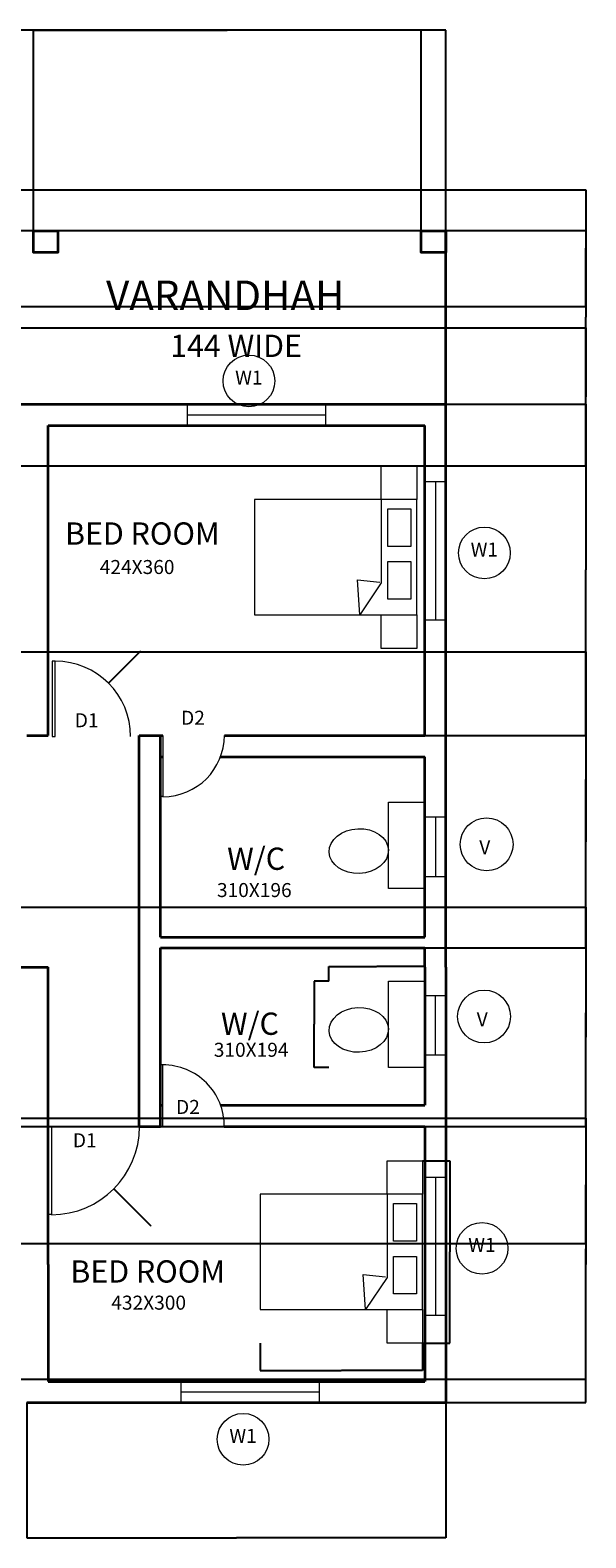
# Model space of a CAD drawing. Units: millimetres. Extents: x -2968 to 14333, y -2966 to 13411.
# Tile 3 of 3: x 8301 to 14333, y -2966 to 13411. Entities that reach past the tile are written whole.
import ezdxf

# ---------------------------------------------------------------- set-up
doc = ezdxf.new("R2010")
doc.units = ezdxf.units.MM
doc.header["$MEASUREMENT"] = 0
for name, color, linetype, lineweight in [('A-ANNO-DIMS', 2, 'Continuous', 18), ('A-ANNO-SYMB', 3, 'Continuous', 13), ('A-AREA-IDEN', 7, 'Continuous', 18), ('A-COLS', 7, 'Continuous', 35), ('A-DOOR', 3, 'Continuous', 18), ('A-FLOR-EDGE', 7, 'Continuous', 25), ('A-FLOR-FIXT', 9, 'Continuous', 18), ('A-FURN', 8, 'Continuous', 18), ('A-GLAZ', 4, 'Continuous', 18), ('A-WALL', 7, 'Continuous', 35)]:
    doc.layers.add(name, color=color, linetype=linetype, lineweight=lineweight)
doc.styles.get("Standard").update_dxf_attribs({"font": 'arial.ttf'})
doc.dimstyles.get("Standard").update_dxf_attribs({"dimtxt": 0.18, "dimasz": 0.18, "dimexe": 0.18, "dimexo": 0.0625, "dimgap": 0.09, "dimtad": 0, "dimtih": 1, "dimtoh": 1, "dimdec": 4, "dimzin": 0, "dimdsep": 46, "dimtxsty": 'Standard', "dimcen": 0.09, "dimadec": 0, "dimazin": 0, "dimtfac": 1, "dimtdec": 4, "dimtofl": 0, "dimtmove": 0, "dimatfit": 3, "dimfxl": 1, "dimtolj": 1, "dimtzin": 0, "dimarcsym": 0})

# ---------------------------------------------------------------- blocks, each defined once
blk = doc.blocks.new('DOOR-SWING-666')
blk.add_lwpolyline([(666.2992070210612, -7.87249337009e-05), (666.2992070210612, 666.0645318323222), (692.9797223629398, 666.0645318323222), (692.9797223629398, -7.87249337009e-05)], close=True)
blk.add_arc((666.2992070210612, -7.87249337009e-05), 666.2995763929106, 90, 180)
blk = doc.blocks.new('WIN-1500')
for p, q in [((-0.0001454069465439, 230.0001364428754), (-0.0001454069465439, 0.0001364428753732)), ((1499.999854593053, 230.0001364428754), (1499.999854593053, 0.0001364428753732)), ((-0.0001454069465439, 115.0001364428753), (1499.999854593053, 115.0001364428753))]:
    blk.add_line(p, q)
blk = doc.blocks.new('WIN-645')
for p, q in [((-0.0001783325678844, 645.3165217330161), (229.9998216674321, 645.3165217330161)), ((114.9998216674321, 645.3165217330161), (114.9998216674321, 9.39247611313e-05)), ((-0.0001783325678844, 9.39247611313e-05), (229.9998216674321, 9.39247611313e-05))]:
    blk.add_line(p, q)
blk = doc.blocks.new('BED-DOUBLE')
for points in [[(1376.583165448723, 1980.905007667385), (1761.472025135164, 1980.905007667385), (1761.472025135164, 1615.931306586089), (1376.583165448723, 1615.931306586089)], [(1761.359434948168, 1616.313451531646), (-6.24364656687e-05, 1616.313451531646), (-6.24364656687e-05, 364.9736316857862), (1761.359434948168, 364.9736316857862)], [(1446.690711967745, 1514.551870762266), (1696.927267861651, 1514.551870762266), (1696.927267861651, 1106.656997559254), (1446.690711967745, 1106.656997559254)], [(1446.690711967745, 942.1830025459176), (1696.927267861651, 942.1830025459176), (1696.927267861651, 534.2881293429062), (1446.690711967745, 534.2881293429062)], [(1376.470575261726, 364.9736316857862), (1761.359434948168, 364.9736316857862), (1761.359434948168, -6.93955107636e-05), (1376.470575261726, -6.93955107636e-05)]]:
    blk.add_lwpolyline(points, close=True)
blk.add_lwpolyline([(1376.583165448723, 1615.931306586089), (1376.583165448723, 711.9201034350671), (1143.773068517777, 363.235888262815), (1117.43252473963, 744.8148033080624), (1361.083249688014, 718.4988451502986)])
blk = doc.blocks.new('WC-PLAN')
blk.add_lwpolyline([(642.4076574105184, 937.925733504826), (1037.697987841055, 937.925733504826), (1037.697987841055, -0.0002773242667899), (642.4076574105184, -0.0002773242667899)], close=True)
blk.add_ellipse((321.2351413435845, 407.2568367539133), major_axis=(321.1725160669339, 12.34114489481309), ratio=0.7569293268408676)
blk = doc.blocks.new('VERANDAH-POST')
blk.add_lwpolyline([(-5.84108229305e-05, 235.3216454025205), (266.2404368537072, 235.3216454025205), (266.2404368537072, -0.0003482651118247), (-5.84108229305e-05, -0.0003482651118247)], close=True)
blk = doc.blocks.new('TAG-V')
blk.add_circle((287.0007825742364, 287.0011250592761), 287.0011736728098)
blk.add_text('V', height=152.3112078732942).set_placement((207.0741385544538, 179.2396726004772))
blk = doc.blocks.new('TAG-W1')
blk.add_circle((280.793431040287, 280.7932079668344), 280.7929963504647)
blk.add_text('W1', height=152.3112078732942).set_placement((130.9915239926576, 241.6268535788358))
blk = doc.blocks.new('*D20')
at = {"layer": 'A-ANNO-DIMS', "color": 0, "lineweight": -2, "transparency": 16777216}
for p, q in [((12560.39380992973, 1130.204523981605), (12857.64707148917, 1130.204523981605)), ((12857.46707148917, 1130.024523981605), (12857.46707148917, 139.9351164187788)), ((12857.46707148917, -850.5205530812917), (12857.46707148917, 139.5688544815346)), ((12560.39380992973, -850.7005530812916), (12857.64707148917, -850.7005530812916))]:
    blk.add_line(p, q, dxfattribs=at)
at = {"layer": 'A-ANNO-DIMS', "color": 0, "transparency": 16777216}
for points in [[(12857.43707148917, 1130.024523981605), (12857.49707148917, 1130.024523981605), (12857.46707148917, 1130.204523981605)], [(12857.43707148917, -850.5205530812917), (12857.49707148917, -850.5205530812917), (12857.46707148917, -850.7005530812916)]]:
    blk.add_solid(points, dxfattribs=at)
at = {"layer": 'Defpoints', "color": 0, "transparency": 16777216}
for p in [(12560.33130992973, 1130.204523981605), (12857.46707148917, 1130.204523981605), (12560.33130992973, -850.7005530812916)]:
    blk.add_point(p, dxfattribs=at)
at = {"layer": 'A-ANNO-DIMS', "color": 0, "transparency": 16777216, "insert": (12857.46707148917, 139.751985450153), "char_height": 0.18, "attachment_point": 5}
blk.add_mtext('\\A1;DOUBLE BED 1981 TYP.', dxfattribs=at)
blk = doc.blocks.new('*D21')
at = {"layer": 'A-ANNO-DIMS', "color": 0, "lineweight": -2, "transparency": 16777216}
for p, q in [((10798.85922235809, -850.7630530812912), (10798.85922235809, -1148.016314640725)), ((12560.33130992972, -850.7630530812912), (12560.33130992972, -1148.016314640725)), ((10799.03922235809, -1147.836314640725), (11678.93579820393, -1147.836314640725)), ((12560.15130992972, -1147.836314640725), (11680.25473408388, -1147.836314640725))]:
    blk.add_line(p, q, dxfattribs=at)
at = {"layer": 'A-ANNO-DIMS', "color": 0, "transparency": 16777216}
for points in [[(10799.03922235809, -1147.806314640725), (10799.03922235809, -1147.866314640725), (10798.85922235809, -1147.836314640725)], [(12560.15130992972, -1147.806314640725), (12560.15130992972, -1147.866314640725), (12560.33130992972, -1147.836314640725)]]:
    blk.add_solid(points, dxfattribs=at)
at = {"layer": 'Defpoints', "color": 0, "transparency": 16777216}
for p in [(10798.85922235809, -850.7005530812913), (12560.33130992972, -850.7005530812913), (12560.33130992972, -1147.836314640725)]:
    blk.add_point(p, dxfattribs=at)
at = {"layer": 'A-ANNO-DIMS', "color": 0, "transparency": 16777216, "insert": (11679.59526614391, -1147.836314640725), "char_height": 0.18, "attachment_point": 5}
blk.add_mtext('\\A1;1761 TYP.', dxfattribs=at)
blk = doc.blocks.new('*D28')
at = {"layer": 'A-ANNO-DIMS', "color": 0, "lineweight": -2, "transparency": 16777216}
for p, q in [((11541.92952659912, 3081.768817646303), (11541.92952659912, 3238.305486832592)), ((11542.10952659912, 3238.125486832593), (12062.41073402773, 3238.125486832593)), ((12584.54398784105, 3238.125486832593), (12064.24278041245, 3238.125486832593)), ((12584.72398784105, 3081.768817646303), (12584.72398784105, 3238.305486832592))]:
    blk.add_line(p, q, dxfattribs=at)
at = {"layer": 'A-ANNO-DIMS', "color": 0, "transparency": 16777216}
for points in [[(11542.10952659912, 3238.155486832593), (11542.10952659912, 3238.095486832592), (11541.92952659912, 3238.125486832593)], [(12584.54398784105, 3238.155486832593), (12584.54398784105, 3238.095486832592), (12584.72398784105, 3238.125486832593)]]:
    blk.add_solid(points, dxfattribs=at)
at = {"layer": 'Defpoints', "color": 0, "transparency": 16777216}
for p in [(12584.72398784105, 3238.125486832593), (11541.92952659912, 3081.706317646303), (12584.72398784105, 3081.706317646303)]:
    blk.add_point(p, dxfattribs=at)
at = {"layer": 'A-ANNO-DIMS', "color": 0, "transparency": 16777216, "insert": (12063.32675722009, 3238.125486832593), "char_height": 0.18, "attachment_point": 5}
blk.add_mtext('\\A1;WC 1043 TYP.', dxfattribs=at)
blk = doc.blocks.new('*D29')
at = {"layer": 'A-ANNO-DIMS', "color": 0, "lineweight": -2, "transparency": 16777216}
for p, q in [((11541.86702659913, 3081.706317646305), (11385.33035741284, 3081.706317646305)), ((11385.51035741284, 3081.526317646305), (11385.51035741284, 2612.925276761089)), ((11385.51035741284, 2143.960306817211), (11385.51035741284, 2612.561347702426)), ((11541.86702659913, 2143.780306817211), (11385.33035741284, 2143.780306817211))]:
    blk.add_line(p, q, dxfattribs=at)
at = {"layer": 'A-ANNO-DIMS', "color": 0, "transparency": 16777216}
for points in [[(11385.48035741284, 3081.526317646305), (11385.54035741284, 3081.526317646305), (11385.51035741284, 3081.706317646305)], [(11385.48035741284, 2143.960306817211), (11385.54035741284, 2143.960306817211), (11385.51035741284, 2143.780306817211)]]:
    blk.add_solid(points, dxfattribs=at)
at = {"layer": 'Defpoints', "color": 0, "transparency": 16777216}
for p in [(11385.51035741284, 3081.706317646305), (11541.92952659913, 3081.706317646305), (11541.92952659913, 2143.780306817211)]:
    blk.add_point(p, dxfattribs=at)
at = {"layer": 'A-ANNO-DIMS', "color": 0, "transparency": 16777216, "insert": (11385.51035741284, 2612.743312231753), "char_height": 0.18, "attachment_point": 5}
blk.add_mtext('\\A1;938 TYP.', dxfattribs=at)
blk = doc.blocks.new('*D32')
at = {"layer": 'A-ANNO-DIMS', "color": 0, "lineweight": -2, "transparency": 16777216}
for p, q in [((-1494.810979, 11907.569973), (-1494.810979, 13410.507299)), ((-1494.630979, 13410.327299), (5659.769102855388, 13410.327299)), ((12815.009021, 13410.327299), (5660.608939144611, 13410.327299)), ((12815.189021, 11235.596939), (12815.189021, 13410.507299))]:
    blk.add_line(p, q, dxfattribs=at)
at = {"layer": 'A-ANNO-DIMS', "color": 0, "transparency": 16777216}
for points in [[(-1494.630979, 13410.357299), (-1494.630979, 13410.297299), (-1494.810979, 13410.327299)], [(12815.009021, 13410.357299), (12815.009021, 13410.297299), (12815.189021, 13410.327299)]]:
    blk.add_solid(points, dxfattribs=at)
at = {"layer": 'Defpoints', "color": 0, "transparency": 16777216}
for p in [(12815.189021, 13410.327299), (-1494.810979, 11907.507473), (12815.189021, 11235.534439)]:
    blk.add_point(p, dxfattribs=at)
at = {"layer": 'A-ANNO-DIMS', "color": 0, "transparency": 16777216, "insert": (5660.189021, 13410.327299), "char_height": 0.18, "attachment_point": 5}
blk.add_mtext('\\A1;14310', dxfattribs=at)
blk = doc.blocks.new('*D36')
at = {"layer": 'A-ANNO-DIMS', "color": 0, "lineweight": -2, "transparency": 16777216}
for p, q in [((8265.189021, -1497.555027), (8265.189021, -2966.059788000001)), ((12815.189021, -1497.555027), (12815.189021, -2966.059788000001)), ((8265.369021, -2965.879788), (10539.82693368758, -2965.879788)), ((12815.009021, -2965.879788), (10540.55110831241, -2965.879788))]:
    blk.add_line(p, q, dxfattribs=at)
at = {"layer": 'A-ANNO-DIMS', "color": 0, "transparency": 16777216}
for points in [[(8265.369021, -2965.849788), (8265.369021, -2965.909788000001), (8265.189021, -2965.879788)], [(12815.009021, -2965.849788), (12815.009021, -2965.909788000001), (12815.189021, -2965.879788)]]:
    blk.add_solid(points, dxfattribs=at)
at = {"layer": 'Defpoints', "color": 0, "transparency": 16777216}
for p in [(8265.189021, -1497.492527), (12815.189021, -1497.492527), (12815.189021, -2965.879788)]:
    blk.add_point(p, dxfattribs=at)
at = {"layer": 'A-ANNO-DIMS', "color": 0, "transparency": 16777216, "insert": (10540.189021, -2965.879788), "char_height": 0.18, "attachment_point": 5}
blk.add_mtext('\\A1;4550', dxfattribs=at)
blk = doc.blocks.new('*D37')
at = {"layer": 'A-ANNO-DIMS', "color": 0, "lineweight": -2, "transparency": 16777216}
for p, q in [((12585.251521, 1502.507473), (14333.28935600001, 1502.507473000001)), ((14333.10935600001, 1502.327473000001), (14333.10935600001, 2.689437529331746)), ((14333.10935600001, -1497.312527), (14333.10935600001, 2.325508470668717)), ((12815.25152100001, -1497.492527), (14333.28935600001, -1497.492527))]:
    blk.add_line(p, q, dxfattribs=at)
at = {"layer": 'A-ANNO-DIMS', "color": 0, "transparency": 16777216}
for points in [[(14333.07935600001, 1502.327473000001), (14333.13935600001, 1502.327473000001), (14333.10935600001, 1502.507473000001)], [(14333.07935600001, -1497.312527), (14333.13935600001, -1497.312527), (14333.10935600001, -1497.492527)]]:
    blk.add_solid(points, dxfattribs=at)
at = {"layer": 'Defpoints', "color": 0, "transparency": 16777216}
for p in [(12585.189021, 1502.507473), (14333.10935600001, 1502.507473000001), (12815.18902100001, -1497.492527)]:
    blk.add_point(p, dxfattribs=at)
at = {"layer": 'A-ANNO-DIMS', "color": 0, "transparency": 16777216, "insert": (14333.10935600001, 2.507472999996171), "char_height": 0.18, "attachment_point": 5}
blk.add_mtext('\\A1;3000', dxfattribs=at)
blk = doc.blocks.new('*D38')
at = {"layer": 'A-ANNO-DIMS', "color": 0, "lineweight": -2, "transparency": 16777216}
for p, q in [((12585.251521, 3442.507473000002), (14333.28935600001, 3442.507473000003)), ((14333.10935600001, 3442.327473000002), (14333.10935600001, 2472.689376137792)), ((14333.10935600001, 1502.687473000001), (14333.10935600001, 2472.325569862212)), ((12585.251521, 1502.507473), (14333.28935600001, 1502.507473000001))]:
    blk.add_line(p, q, dxfattribs=at)
at = {"layer": 'A-ANNO-DIMS', "color": 0, "transparency": 16777216}
for points in [[(14333.07935600001, 3442.327473000002), (14333.13935600001, 3442.327473000002), (14333.10935600001, 3442.507473000003)], [(14333.07935600001, 1502.687473000001), (14333.13935600001, 1502.687473000001), (14333.10935600001, 1502.507473000001)]]:
    blk.add_solid(points, dxfattribs=at)
at = {"layer": 'Defpoints', "color": 0, "transparency": 16777216}
for p in [(12585.189021, 3442.507473000002), (14333.10935600001, 3442.507473000003), (12585.189021, 1502.507473)]:
    blk.add_point(p, dxfattribs=at)
at = {"layer": 'A-ANNO-DIMS', "color": 0, "transparency": 16777216, "insert": (14333.10935600001, 2472.507472999997), "char_height": 0.18, "attachment_point": 5}
blk.add_mtext('\\A1;1940', dxfattribs=at)
blk = doc.blocks.new('*D39')
at = {"layer": 'A-ANNO-DIMS', "color": 0, "lineweight": -2, "transparency": 16777216}
for p, q in [((12585.251521, 5747.507473000002), (14333.28935600001, 5747.507473000002)), ((14333.10935600001, 5747.327473000002), (14333.10935600001, 4595.189437529334)), ((14333.10935600002, 3442.687473000002), (14333.10935600001, 4594.82550847067)), ((12585.251521, 3442.507473000002), (14333.28935600002, 3442.507473000003))]:
    blk.add_line(p, q, dxfattribs=at)
at = {"layer": 'A-ANNO-DIMS', "color": 0, "transparency": 16777216}
for points in [[(14333.07935600001, 5747.327473000002), (14333.13935600001, 5747.327473000002), (14333.10935600001, 5747.507473000002)], [(14333.07935600002, 3442.687473000002), (14333.13935600001, 3442.687473000002), (14333.10935600002, 3442.507473000003)]]:
    blk.add_solid(points, dxfattribs=at)
at = {"layer": 'Defpoints', "color": 0, "transparency": 16777216}
for p in [(12585.189021, 5747.507473000002), (14333.10935600001, 5747.507473000002), (12585.189021, 3442.507473000002)]:
    blk.add_point(p, dxfattribs=at)
at = {"layer": 'A-ANNO-DIMS', "color": 0, "transparency": 16777216, "insert": (14333.10935600001, 4595.007472999997), "char_height": 0.18, "attachment_point": 5}
blk.add_mtext('\\A1;2305', dxfattribs=at)
blk = doc.blocks.new('*D40')
at = {"layer": 'A-ANNO-DIMS', "color": 0, "lineweight": -2, "transparency": 16777216}
for p, q in [((12815.25152100001, 9347.507473000003), (14333.28935600001, 9347.507473000003)), ((14333.10935600001, 9347.327473000003), (14333.10935600001, 7547.689437529334)), ((14333.10935600001, 5747.687473000002), (14333.10935600001, 7547.32550847067)), ((12585.251521, 5747.507473000002), (14333.28935600001, 5747.507473000002))]:
    blk.add_line(p, q, dxfattribs=at)
at = {"layer": 'A-ANNO-DIMS', "color": 0, "transparency": 16777216}
for points in [[(14333.07935600001, 9347.327473000003), (14333.13935600001, 9347.327473000003), (14333.10935600001, 9347.507473000003)], [(14333.07935600001, 5747.687473000002), (14333.13935600001, 5747.687473000002), (14333.10935600001, 5747.507473000002)]]:
    blk.add_solid(points, dxfattribs=at)
at = {"layer": 'Defpoints', "color": 0, "transparency": 16777216}
for p in [(12815.18902100001, 9347.507473000003), (14333.10935600001, 9347.507473000003), (12585.189021, 5747.507473000002)]:
    blk.add_point(p, dxfattribs=at)
at = {"layer": 'A-ANNO-DIMS', "color": 0, "transparency": 16777216, "insert": (14333.10935600001, 7547.507472999997), "char_height": 0.18, "attachment_point": 5}
blk.add_mtext('\\A1;3600', dxfattribs=at)
blk = doc.blocks.new('*D41')
at = {"layer": 'A-ANNO-DIMS', "color": 0, "lineweight": -2, "transparency": 16777216}
for p, q in [((12815.25152100001, 11235.534439), (14333.28935600001, 11235.534439)), ((14333.10935600001, 11235.354439), (14333.10935600001, 10291.70285913779)), ((14333.10935600001, 9347.687473000004), (14333.10935600001, 10291.33905286221)), ((12815.25152100001, 9347.507473000003), (14333.28935600001, 9347.507473000003))]:
    blk.add_line(p, q, dxfattribs=at)
at = {"layer": 'A-ANNO-DIMS', "color": 0, "transparency": 16777216}
for points in [[(14333.07935600001, 11235.354439), (14333.13935600001, 11235.354439), (14333.10935600001, 11235.534439)], [(14333.07935600001, 9347.687473000004), (14333.13935600001, 9347.687473000004), (14333.10935600001, 9347.507473000003)]]:
    blk.add_solid(points, dxfattribs=at)
at = {"layer": 'Defpoints', "color": 0, "transparency": 16777216}
for p in [(12815.18902100001, 11235.534439), (14333.10935600001, 11235.534439), (12815.18902100001, 9347.507473000003)]:
    blk.add_point(p, dxfattribs=at)
at = {"layer": 'A-ANNO-DIMS', "color": 0, "transparency": 16777216, "insert": (14333.10935600001, 10291.52095599999), "char_height": 0.18, "attachment_point": 5}
blk.add_mtext('\\A1;1888', dxfattribs=at)
blk = doc.blocks.new('*D47')
at = {"layer": 'A-ANNO-DIMS', "color": 0, "lineweight": -2, "transparency": 16777216}
for p, q in [((-1264.748479, 11677.507473), (14333.28935600001, 11677.507473)), ((14333.10935600001, 11677.327473), (14333.10935600001, 11042.68937613779)), ((14333.10935600001, 10407.687473), (14333.10935600001, 11042.32556986221)), ((-1264.748479, 10407.507473), (14333.28935600001, 10407.507473))]:
    blk.add_line(p, q, dxfattribs=at)
at = {"layer": 'A-ANNO-DIMS', "color": 0, "transparency": 16777216}
for points in [[(14333.07935600001, 11677.327473), (14333.13935600001, 11677.327473), (14333.10935600001, 11677.507473)], [(14333.07935600001, 10407.687473), (14333.13935600001, 10407.687473), (14333.10935600001, 10407.507473)]]:
    blk.add_solid(points, dxfattribs=at)
at = {"layer": 'Defpoints', "color": 0, "transparency": 16777216}
for p in [(-1264.810979000001, 11677.507473), (14333.10935600001, 11677.507473), (-1264.810979000001, 10407.507473)]:
    blk.add_point(p, dxfattribs=at)
at = {"layer": 'A-ANNO-DIMS', "color": 0, "transparency": 16777216, "insert": (14333.10935600001, 11042.507473), "char_height": 0.18, "attachment_point": 5}
blk.add_mtext('\\A1;1270', dxfattribs=at)
blk = doc.blocks.new('*D51')
at = {"layer": 'A-ANNO-DIMS', "color": 0, "lineweight": -2, "transparency": 16777216}
for p, q in [((6227.180942, 11232.243145), (6227.180942, 13410.507299)), ((6227.360942, 13410.327299), (7281.505338680763, 13410.327299)), ((8336.57994, 13410.327299), (7282.435543319237, 13410.327299)), ((8336.75994, 11232.243145), (8336.75994, 13410.507299))]:
    blk.add_line(p, q, dxfattribs=at)
at = {"layer": 'A-ANNO-DIMS', "color": 0, "transparency": 16777216}
for points in [[(6227.360942, 13410.357299), (6227.360942, 13410.297299), (6227.180942, 13410.327299)], [(8336.57994, 13410.357299), (8336.57994, 13410.297299), (8336.75994, 13410.327299)]]:
    blk.add_solid(points, dxfattribs=at)
at = {"layer": 'Defpoints', "color": 0, "transparency": 16777216}
for p in [(8336.75994, 13410.327299), (6227.180942, 11232.180645), (8336.75994, 11232.180645)]:
    blk.add_point(p, dxfattribs=at)
at = {"layer": 'A-ANNO-DIMS', "color": 0, "transparency": 16777216, "insert": (7281.970441, 13410.327299), "char_height": 0.18, "attachment_point": 5}
blk.add_mtext('\\A1;2109.6', dxfattribs=at)
blk = doc.blocks.new('*D52')
at = {"layer": 'A-ANNO-DIMS', "color": 0, "lineweight": -2, "transparency": 16777216}
for p, q in [((8336.75994, 11232.243145), (8336.75994, 13410.507299)), ((8336.93994, 13410.327299), (10440.85984355525, 13410.327299)), ((12545.504904, 13410.327299), (10441.58500044474, 13410.327299)), ((12545.684904, 11232.243145), (12545.684904, 13410.507299))]:
    blk.add_line(p, q, dxfattribs=at)
at = {"layer": 'A-ANNO-DIMS', "color": 0, "transparency": 16777216}
for points in [[(8336.93994, 13410.357299), (8336.93994, 13410.297299), (8336.75994, 13410.327299)], [(12545.504904, 13410.357299), (12545.504904, 13410.297299), (12545.684904, 13410.327299)]]:
    blk.add_solid(points, dxfattribs=at)
at = {"layer": 'Defpoints', "color": 0, "transparency": 16777216}
for p in [(12545.684904, 13410.327299), (8336.75994, 11232.180645), (12545.684904, 11232.180645)]:
    blk.add_point(p, dxfattribs=at)
at = {"layer": 'A-ANNO-DIMS', "color": 0, "transparency": 16777216, "insert": (10441.222422, 13410.327299), "char_height": 0.18, "attachment_point": 5}
blk.add_mtext('\\A1;4209', dxfattribs=at)
blk = doc.blocks.new('*D53')
at = {"layer": 'A-ANNO-DIMS', "color": 0, "lineweight": -2, "transparency": 16777216}
for p, q in [((-1220.345468, 1592.680140000001), (14333.28935600001, 1592.680140000003)), ((14333.10935600001, 1592.500140000003), (14333.10935600001, 175.1113265293341)), ((14333.10935600001, -1242.641415999998), (14333.10935600001, 174.7473974706711)), ((-1236.815201, -1242.821416), (14333.28935600001, -1242.821415999998))]:
    blk.add_line(p, q, dxfattribs=at)
at = {"layer": 'A-ANNO-DIMS', "color": 0, "transparency": 16777216}
for points in [[(14333.07935600001, 1592.500140000003), (14333.13935600001, 1592.500140000003), (14333.10935600001, 1592.680140000003)], [(14333.07935600001, -1242.641415999998), (14333.13935600001, -1242.641415999998), (14333.10935600001, -1242.821415999998)]]:
    blk.add_solid(points, dxfattribs=at)
at = {"layer": 'Defpoints', "color": 0, "transparency": 16777216}
for p in [(-1220.407968, 1592.680140000001), (14333.10935600001, 1592.680140000003), (-1236.877701, -1242.821416)]:
    blk.add_point(p, dxfattribs=at)
at = {"layer": 'A-ANNO-DIMS', "color": 0, "transparency": 16777216, "insert": (14333.10935600001, 174.9293619999985), "char_height": 0.18, "attachment_point": 5}
blk.add_mtext('\\A1;2835.5', dxfattribs=at)
blk = doc.blocks.new('*D54')
at = {"layer": 'A-ANNO-DIMS', "color": 0, "lineweight": -2, "transparency": 16777216}
for p, q in [((-1220.345468, 3884.149375000002), (14333.28935600001, 3884.149375000005)), ((14333.10935600001, 3883.969375000005), (14333.10935600001, 2738.596660637794)), ((14333.10935600001, 1592.860140000003), (14333.10935600001, 2738.232854362214)), ((-1220.345468, 1592.680140000001), (14333.28935600001, 1592.680140000003))]:
    blk.add_line(p, q, dxfattribs=at)
at = {"layer": 'A-ANNO-DIMS', "color": 0, "transparency": 16777216}
for points in [[(14333.07935600001, 3883.969375000005), (14333.13935600001, 3883.969375000005), (14333.10935600001, 3884.149375000005)], [(14333.07935600001, 1592.860140000003), (14333.13935600001, 1592.860140000003), (14333.10935600001, 1592.680140000003)]]:
    blk.add_solid(points, dxfattribs=at)
at = {"layer": 'Defpoints', "color": 0, "transparency": 16777216}
for p in [(-1220.407968, 3884.149375000002), (14333.10935600001, 3884.149375000005), (-1220.407968, 1592.680140000001)]:
    blk.add_point(p, dxfattribs=at)
at = {"layer": 'A-ANNO-DIMS', "color": 0, "transparency": 16777216, "insert": (14333.10935600001, 2738.414757499999), "char_height": 0.18, "attachment_point": 5}
blk.add_mtext('\\A1;2291.5', dxfattribs=at)
blk = doc.blocks.new('*D55')
at = {"layer": 'A-ANNO-DIMS', "color": 0, "lineweight": -2, "transparency": 16777216}
for p, q in [((-1494.748479, 6657.507473000004), (14333.28935600001, 6657.507473000006)), ((14333.10935600001, 6657.327473000005), (14333.10935600001, 5271.010388529336)), ((14333.10935600002, 3884.329375000005), (14333.10935600001, 5270.646459470672)), ((-1220.345468, 3884.149375000002), (14333.28935600002, 3884.149375000005))]:
    blk.add_line(p, q, dxfattribs=at)
at = {"layer": 'A-ANNO-DIMS', "color": 0, "transparency": 16777216}
for points in [[(14333.07935600001, 6657.327473000005), (14333.13935600001, 6657.327473000005), (14333.10935600001, 6657.507473000006)], [(14333.07935600002, 3884.329375000005), (14333.13935600001, 3884.329375000005), (14333.10935600002, 3884.149375000005)]]:
    blk.add_solid(points, dxfattribs=at)
at = {"layer": 'Defpoints', "color": 0, "transparency": 16777216}
for p in [(-1494.810979, 6657.507473000004), (14333.10935600001, 6657.507473000006), (-1220.407968, 3884.149375000002)]:
    blk.add_point(p, dxfattribs=at)
at = {"layer": 'A-ANNO-DIMS', "color": 0, "transparency": 16777216, "insert": (14333.10935600001, 5270.828424), "char_height": 0.18, "attachment_point": 5}
blk.add_mtext('\\A1;2773.4', dxfattribs=at)
blk = doc.blocks.new('*D61')
at = {"layer": 'A-ANNO-DIMS', "color": 0, "lineweight": -2, "transparency": 16777216}
for p, q in [((1505.251521, 10177.507473), (14333.28935600001, 10177.507473)), ((14333.10935600001, 10177.327473), (14333.10935600001, 9427.689376137798)), ((14333.10935600001, 8677.687473000007), (14333.10935600001, 9427.325569862218)), ((1505.251521, 8677.507473000003), (14333.28935600001, 8677.507473000007))]:
    blk.add_line(p, q, dxfattribs=at)
at = {"layer": 'A-ANNO-DIMS', "color": 0, "transparency": 16777216}
for points in [[(14333.07935600001, 10177.327473), (14333.13935600001, 10177.327473), (14333.10935600001, 10177.507473)], [(14333.07935600001, 8677.687473000007), (14333.13935600001, 8677.687473000007), (14333.10935600001, 8677.507473000007)]]:
    blk.add_solid(points, dxfattribs=at)
at = {"layer": 'Defpoints', "color": 0, "transparency": 16777216}
for p in [(1505.189021, 10177.507473), (14333.10935600001, 10177.507473), (1505.189021, 8677.507473000003)]:
    blk.add_point(p, dxfattribs=at)
at = {"layer": 'A-ANNO-DIMS', "color": 0, "transparency": 16777216, "insert": (14333.10935600001, 9427.507473000001), "char_height": 0.18, "attachment_point": 5}
blk.add_mtext('\\A1;1500', dxfattribs=at)
blk = doc.blocks.new('*D62')
at = {"layer": 'A-ANNO-DIMS', "color": 0, "lineweight": -2, "transparency": 16777216}
for p, q in [((235.2515210000001, 1502.507473), (14333.28935600001, 1502.507473000003)), ((14333.10935600001, 1502.327473000002), (14333.10935600001, 867.6893761377925)), ((14333.10935600001, 232.6874730000024), (14333.10935600001, 867.3255698622125)), ((235.2515210000001, 232.5074730000001), (14333.28935600001, 232.5074730000024))]:
    blk.add_line(p, q, dxfattribs=at)
at = {"layer": 'A-ANNO-DIMS', "color": 0, "transparency": 16777216}
for points in [[(14333.07935600001, 1502.327473000002), (14333.13935600001, 1502.327473000002), (14333.10935600001, 1502.507473000003)], [(14333.07935600001, 232.6874730000024), (14333.13935600001, 232.6874730000024), (14333.10935600001, 232.5074730000024)]]:
    blk.add_solid(points, dxfattribs=at)
at = {"layer": 'Defpoints', "color": 0, "transparency": 16777216}
for p in [(235.1890210000001, 1502.507473), (14333.10935600001, 1502.507473000003), (235.1890210000001, 232.5074730000001)]:
    blk.add_point(p, dxfattribs=at)
at = {"layer": 'A-ANNO-DIMS', "color": 0, "transparency": 16777216, "insert": (14333.10935600001, 867.5074729999982), "char_height": 0.18, "attachment_point": 5}
blk.add_mtext('\\A1;1270', dxfattribs=at)
blk = doc.blocks.new('*D63')
at = {"layer": 'A-ANNO-DIMS', "color": 0, "lineweight": -2, "transparency": 16777216}
for p, q in [((8532.343252999997, 1500.324317999999), (8532.523253, 1500.324318)), ((8532.433252999997, 1500.234318), (8532.433252999997, 1500.414318)), ((9614.330248214712, 418.4280091852897), (9208.746154260987, 824.0118458197621)), ((9614.510248214712, 418.4280091852888), (9614.330248214712, 418.4280091852897))]:
    blk.add_line(p, q, dxfattribs=at)
at = {"layer": 'A-ANNO-DIMS', "color": 0, "transparency": 16777216}
blk.add_solid([(9208.767367457694, 824.0330590299272), (9208.72494106428, 823.9906326095979), (9208.618874999996, 824.1391249999997)], dxfattribs=at)
at = {"layer": 'Defpoints', "color": 0, "transparency": 16777216}
for p in [(8532.433252999997, 1500.324317999999), (9208.618874999996, 824.1391249999997)]:
    blk.add_point(p, dxfattribs=at)
at = {"layer": 'A-ANNO-DIMS', "color": 0, "transparency": 16777216, "insert": (9614.990084503936, 418.4280091852888), "char_height": 0.18, "attachment_point": 5}
blk.add_mtext('\\A1;R956.3', dxfattribs=at)
blk = doc.blocks.new('*D64')
at = {"layer": 'A-ANNO-DIMS', "color": 0, "lineweight": -2, "transparency": 16777216}
for p, q in [((9499.39044289954, 6663.641486099539), (9152.0529512127, 6316.303951228529)), ((9499.57044289954, 6663.641486099539), (9499.39044289954, 6663.641486099539)), ((8572.727719999999, 5737.068648000001), (8572.90772, 5737.068648000002)), ((8572.81772, 5736.978648000001), (8572.81772, 5737.158648000002))]:
    blk.add_line(p, q, dxfattribs=at)
at = {"layer": 'A-ANNO-DIMS', "color": 0, "transparency": 16777216}
blk.add_solid([(9152.031738007947, 6316.325164430645), (9152.074164417456, 6316.282738026412), (9151.925672000001, 6316.176672000001)], dxfattribs=at)
at = {"layer": 'Defpoints', "color": 0, "transparency": 16777216}
for p in [(9151.925672000001, 6316.176672000001), (8572.81772, 5737.068648000001)]:
    blk.add_point(p, dxfattribs=at)
at = {"layer": 'A-ANNO-DIMS', "color": 0, "transparency": 16777216, "insert": (9499.945606610318, 6663.641486099539), "char_height": 0.18, "attachment_point": 5}
blk.add_mtext('\\A1;R819', dxfattribs=at)

msp = doc.modelspace()

# ---------------------------------------------------------------- linework, layer by layer
at = {"layer": 'A-DOOR'}
for points in [[(8572.817719924968, 5737.06864835125), (8572.817719924968, 6555.76221037819), (8540.02335464007, 6555.76221037819), (8540.02335464007, 5737.06864835125)], [(9742.184979406316, 1505.596455822391), (9742.184979406316, 2171.661066379647), (9715.504464064437, 2171.661066379647), (9715.504464064437, 1505.596455822391)], [(8532.433252793688, 1500.324317739224), (8532.433252793688, 544.3909657900787), (8494.14148040669, 544.3909657900787), (8494.14148040669, 1500.324317739224)]]:
    msp.add_lwpolyline(points, close=True, dxfattribs=at)
for centre, radius, start, end in [((8572.817719924968, 5737.06864835125), 818.9823703706011, 0, 90), ((9742.184979406316, 1505.596455822391), 666.2995763929106, 359.7343742993682, 90), ((8532.433252793688, 1500.324317739224), 956.270574007352, 270, 0)]:
    msp.add_arc(centre, radius, start, end, dxfattribs=at)
at = {"layer": 'A-FLOR-EDGE'}
msp.add_line((3005.189021442665, 11235.53443915362), (12815.18902144266, 11235.53443915362), dxfattribs=at)
at = {"layer": 'A-WALL'}
for p, q in [((12815.18902144266, 3232.507473364635), (12815.18902144266, 11235.53443915362)), ((3943.020669778164, 9347.507473364634), (12815.18902144266, 9347.507473364634)), ((8495.189021442664, 5747.507473364635), (8495.189021442664, 9117.507473364634)), ((8495.189021442664, 9117.507473364634), (12585.18902144266, 9117.507473364634)), ((12585.18902144266, 5747.507473364635), (12585.18902144265, 9117.507473364634)), ((12585.18902144266, 6887.507473364635), (12585.18902144266, 9117.507473364634)), ((8265.189021442662, 5747.507473364635), (8495.189021442664, 5747.507473364635)), ((9485.18902144266, 1502.507473364634), (9485.189021442664, 5747.507473364635)), ((9485.189021442664, 5747.507473364635), (9743.006470771405, 5747.507473364635)), ((9715.189021442662, 3557.507473364636), (9715.189021442662, 5747.507473364635)), ((10409.29821703777, 5747.507473364635), (12585.18902144266, 5747.507473364635)), ((9715.189021442666, 5517.507473364635), (9743.006470771405, 5517.507473364635)), ((10367.15291775114, 5517.507473364635), (12585.18902144266, 5517.507473364634)), ((12585.18902144266, 3557.507473364634), (12585.18902144266, 5517.507473364634)), ((9715.189021442662, 3557.507473364635), (12585.18902144266, 3557.507473364635)), ((9715.18902144266, 1502.507473364634), (9715.189021442662, 3442.507473364635)), ((9715.189021442662, 3442.507473364635), (12585.18902144266, 3442.507473364634)), ((12585.18902144266, 3232.507473364635), (12585.18902144266, 3442.507473364634)), ((4530.982965129427, 3232.507473364635), (8495.189021442664, 3232.507473364635)), ((8495.189021442664, 2.507473364634584), (8495.189021442664, 3232.507473364635)), ((12585.18902144266, 3232.507473364635), (12585.18902144266, 1732.507473364634)), ((12815.18902144266, 3232.507473364635), (12815.18902144266, -1497.492526635365)), ((9715.18902144266, 1732.507473364634), (9742.184979406316, 1732.507473364634)), ((10368.65645969837, 1732.507473364634), (12585.18902144266, 1732.507473364634)), ((9485.18902144266, 1502.507473364634), (9715.18902144266, 1502.507473364634)), ((10408.47739545857, 1502.507473364634), (12585.18902144266, 1502.507473364634)), ((12585.18902144266, 1502.507473364634), (12585.18902144266, -1267.492526635365)), ((8495.189021442664, 2.507473364634584), (8495.189021442664, -1267.492526635365)), ((8495.189021442664, -1267.492526635365), (12585.18902144266, -1267.492526635365)), ((8265.189021442662, -1497.492526635365), (12815.18902144266, -1497.492526635365))]:
    msp.add_line(p, q, dxfattribs=at)

# ---------------------------------------------------------------- block references
at = {"layer": 'A-ANNO-SYMB'}
for name, p in [('TAG-W1', (10395.15295692121, 9319.31206343592)), ('TAG-W1', (12951.89730814433, 7450.813546891217)), ('TAG-V', (12969.6073993196, 4279.860557452579)), ('TAG-V', (12941.69362440456, 2410.109753944717)), ('TAG-W1', (12925.9211488325, -102.1825538586081)), ('TAG-W1', (10332.241, -2176.38))]:
    msp.add_blockref(name, p, dxfattribs=at)
at = {"layer": 'A-COLS'}
for p in [(8336.759998140991, 10996.859), (12545.68496197289, 10996.859)]:
    msp.add_blockref('VERANDAH-POST', p, dxfattribs=at)
at = {"layer": 'A-DOOR', "rotation": 180}
msp.add_blockref('DOOR-SWING-666', (10409.30567779246, 5750.737620433749), dxfattribs=at)
at = {"layer": 'A-FLOR-FIXT'}
for p in [(11547.026, 4086.661), (11547.026, 2143.780584141477)]:
    msp.add_blockref('WC-PLAN', p, dxfattribs=at)
at = {"layer": 'A-FURN'}
for p in [(10735.806, 6695.488), (10798.85928479456, -850.7004836857805)]:
    msp.add_blockref('BED-DOUBLE', p, dxfattribs=at)
at = {"layer": 'A-GLAZ'}
for name, p in [('WIN-1500', (10006.07016014705, 9117.562812091104)), ('WIN-645', (12585.164, 4219.243999999999)), ('WIN-1500', (9937.910006864711, -1496.857030888883))]:
    msp.add_blockref(name, p, dxfattribs=at)
for name, p, rotation in [('WIN-1500', (12584.70110934981, 8503.578124491421), 269.9999999999997), ('WIN-645', (12815.89024918978, 2921.529433536291), 180), ('WIN-1500', (12585.38499048639, 949.6600034178506), 270.0000000000002)]:
    msp.add_blockref(name, p, dxfattribs=dict(at, rotation=rotation))

# ---------------------------------------------------------------- texts
at = {"layer": 'A-ANNO-SYMB'}
for s, p in [('D1', (8785.62070646882, 5838.192045941949)), ('D2', (9939.652455195785, 5865.634403403849)), ('D2', (9884.733162678776, 1638.107929624617)), ('D1', (8764.609687171876, 1276.175405554473))]:
    msp.add_text(s, height=152.3112078732942, dxfattribs=at).set_placement(p)
at = {"layer": 'A-AREA-IDEN'}
for s, height, p in [('VARANDHAH', 321.4922915585339, (9124.885090127587, 10369.03105913102)), ('144 WIDE', 241.7589680836474, (9820.887379232076, 9860.484654800153)), ('BED ROOM', 241.7589680836474, (8679.692333939696, 7822.020569474553)), ('424X360', 152.3112078732942, (9056.702551870932, 7502.99975043192)), ('W/C', 241.7589680836474, (10439.28951207104, 4289.79404633597)), ('310X196', 152.3112078732942, (10328.98940344839, 3993.983718455131)), ('W/C', 241.7589680836474, (10372.44177343997, 2497.512305424665)), ('310X194', 152.3112078732942, (10294.59672632753, 2258.961719464803)), ('BED ROOM', 241.7589680836474, (8737.518049876417, -193.5228356447769)), ('432X300', 152.3112078732942, (9182.102612293653, -487.5626888495735))]:
    msp.add_text(s, height=height, dxfattribs=at).set_placement(p)

# ---------------------------------------------------------------- dimensions: what is measured, and where the dimension line sits
at = {"layer": 'A-ANNO-DIMS'}
for base, p1, p2, override, picture, middle in [((12815.189021, 13410.327299), (-1494.810979, 11907.507473), (12815.189021, 11235.534439), {"dimdec": 0, "dimlfac": 1, "dimrnd": 0, "dimzin": 0, "dimdsep": 46, "dimlunit": 2}, '*D32', (5660.189021, 13410.327299)), ((8336.75994, 13410.327299), (6227.180942, 11232.180645), (8336.75994, 11232.180645), {"dimdec": 1, "dimlfac": 1, "dimrnd": 0, "dimzin": 0, "dimdsep": 46, "dimlunit": 2}, '*D51', (7281.970441, 13410.327299)), ((12545.684904, 13410.327299), (8336.75994, 11232.180645), (12545.684904, 11232.180645), {"dimdec": 0, "dimlfac": 1, "dimrnd": 0, "dimzin": 0, "dimdsep": 46, "dimlunit": 2}, '*D52', (10441.222422, 13410.327299)), ((12815.189021, -2965.879788), (8265.189021, -1497.492527), (12815.189021, -1497.492527), {"dimdec": 0, "dimlfac": 1, "dimrnd": 0, "dimzin": 0, "dimdsep": 46, "dimlunit": 2}, '*D36', (10540.189021, -2965.879788))]:
    dim = msp.add_linear_dim(base=base, p1=p1, p2=p2, dimstyle='Standard', override=override, dxfattribs=at)
    dim.commit()
    dim.dimension.update_dxf_attribs({"geometry": picture, "text_midpoint": middle})
for base, p1, p2, override, picture, middle in [((14333.10935600001, 11677.507473), (-1264.810979, 10407.507473), (-1264.810979, 11677.507473), {"dimdec": 0, "dimlfac": 1, "dimrnd": 0, "dimzin": 0, "dimdsep": 46, "dimlunit": 2}, '*D47', (14333.10935600001, 11042.507473)), ((14333.10935600001, 11235.534439), (12815.189021, 9347.507473), (12815.189021, 11235.534439), {"dimdec": 0, "dimlfac": 1, "dimrnd": 0, "dimzin": 0, "dimdsep": 46, "dimlunit": 2}, '*D41', (14333.10935600001, 10291.52095599999)), ((14333.10935600001, 10177.507473), (1505.189021, 8677.507473), (1505.189021, 10177.507473), {"dimdec": 0, "dimlfac": 1, "dimrnd": 0, "dimzin": 0, "dimdsep": 46, "dimlunit": 2}, '*D61', (14333.10935600001, 9427.507473000001)), ((14333.10935600001, 9347.507473000003), (12585.189021, 5747.507472999999), (12815.189021, 9347.507473), {"dimdec": 0, "dimlfac": 1, "dimrnd": 0, "dimzin": 0, "dimdsep": 46, "dimlunit": 2}, '*D40', (14333.10935600001, 7547.507472999997)), ((14333.10935600001, 6657.507473000006), (-1220.407968, 3884.149375), (-1494.810979, 6657.507472999999), {"dimdec": 1, "dimlfac": 1, "dimrnd": 0, "dimzin": 0, "dimdsep": 46, "dimlunit": 2}, '*D55', (14333.10935600001, 5270.828424)), ((14333.10935600001, 5747.507473000002), (12585.189021, 3442.507473), (12585.189021, 5747.507472999999), {"dimdec": 0, "dimlfac": 1, "dimrnd": 0, "dimzin": 0, "dimdsep": 46, "dimlunit": 2}, '*D39', (14333.10935600001, 4595.007472999997)), ((14333.10935600001, 3884.149375000005), (-1220.407968, 1592.68014), (-1220.407968, 3884.149375), {"dimdec": 1, "dimlfac": 1, "dimrnd": 0, "dimzin": 0, "dimdsep": 46, "dimlunit": 2}, '*D54', (14333.10935600001, 2738.414757499999)), ((14333.10935600001, 3442.507473000003), (12585.189021, 1502.507473), (12585.189021, 3442.507473), {"dimdec": 0, "dimlfac": 1, "dimrnd": 0, "dimzin": 0, "dimdsep": 46, "dimlunit": 2}, '*D38', (14333.10935600001, 2472.507472999997)), ((14333.10935600001, 1592.680140000003), (-1236.877701, -1242.821416), (-1220.407968, 1592.68014), {"dimdec": 1, "dimlfac": 1, "dimrnd": 0, "dimzin": 0, "dimdsep": 46, "dimlunit": 2}, '*D53', (14333.10935600001, 174.9293619999985)), ((14333.10935600001, 1502.507473000003), (235.189021, 232.507473), (235.189021, 1502.507473), {"dimdec": 0, "dimlfac": 1, "dimrnd": 0, "dimzin": 0, "dimdsep": 46, "dimlunit": 2}, '*D62', (14333.10935600001, 867.5074729999982)), ((14333.10935600001, 1502.507473000001), (12815.189021, -1497.492527), (12585.189021, 1502.507473), {"dimdec": 0, "dimlfac": 1, "dimrnd": 0, "dimzin": 0, "dimdsep": 46, "dimlunit": 2}, '*D37', (14333.10935600001, 2.507472999996171))]:
    dim = msp.add_linear_dim(base=base, p1=p1, p2=p2, angle=90, dimstyle='Standard', override=override, dxfattribs=at)
    dim.commit()
    dim.dimension.update_dxf_attribs({"geometry": picture, "text_midpoint": middle})
for center, mpoint, override, picture, middle in [((8572.81772, 5737.068648000001), (9151.925672000001, 6316.176672000001), {"dimdec": 0, "dimlfac": 1, "dimrnd": 0, "dimzin": 0, "dimdsep": 46, "dimlunit": 2}, '*D64', (9499.945606610318, 6663.641486099539)), ((8532.433252999997, 1500.324317999999), (9208.618874999996, 824.1391249999997), {"dimdec": 1, "dimlfac": 1, "dimrnd": 0, "dimzin": 0, "dimdsep": 46, "dimlunit": 2}, '*D63', (9614.990084503936, 418.4280091852888))]:
    dim = msp.add_radius_dim(center=center, mpoint=mpoint, dimstyle='Standard', override=override, dxfattribs=at)
    dim.commit()
    dim.dimension.update_dxf_attribs({"geometry": picture, "text_midpoint": middle, "dimtype": 164})
for base, p1, p2, text, picture, middle in [((12584.72398784105, 3238.125486832593), (11541.92952659912, 3081.706317646303), (12584.72398784105, 3081.706317646303), 'WC <> TYP.', '*D28', (12063.32675722009, 3238.125486832593)), ((12560.33130992972, -1147.836314640725), (10798.85922235809, -850.7005530812913), (12560.33130992972, -850.7005530812913), '<> TYP.', '*D21', (11679.59526614391, -1147.836314640725))]:
    dim = msp.add_linear_dim(base=base, p1=p1, p2=p2, text=text, dimstyle='Standard', override={"dimdec": 0, "dimlfac": 1, "dimrnd": 0, "dimzin": 0, "dimdsep": 46, "dimlunit": 2}, dxfattribs=at)
    dim.commit()
    dim.dimension.update_dxf_attribs({"geometry": picture, "text_midpoint": middle})
for base, p1, p2, text, picture, middle in [((11385.51035741284, 3081.706317646305), (11541.92952659912, 2143.78030681721), (11541.92952659912, 3081.706317646303), '<> TYP.', '*D29', (11385.51035741284, 2612.743312231753)), ((12857.46707148917, 1130.204523981605), (12560.33130992972, -850.7005530812913), (12560.33130992972, 1130.204523981604), 'DOUBLE BED <> TYP.', '*D20', (12857.46707148917, 139.751985450153))]:
    dim = msp.add_linear_dim(base=base, p1=p1, p2=p2, angle=90, text=text, dimstyle='Standard', override={"dimdec": 0, "dimlfac": 1, "dimrnd": 0, "dimzin": 0, "dimdsep": 46, "dimlunit": 2}, dxfattribs=at)
    dim.commit()
    dim.dimension.update_dxf_attribs({"geometry": picture, "text_midpoint": middle})

doc.saveas('drawing.dxf')
